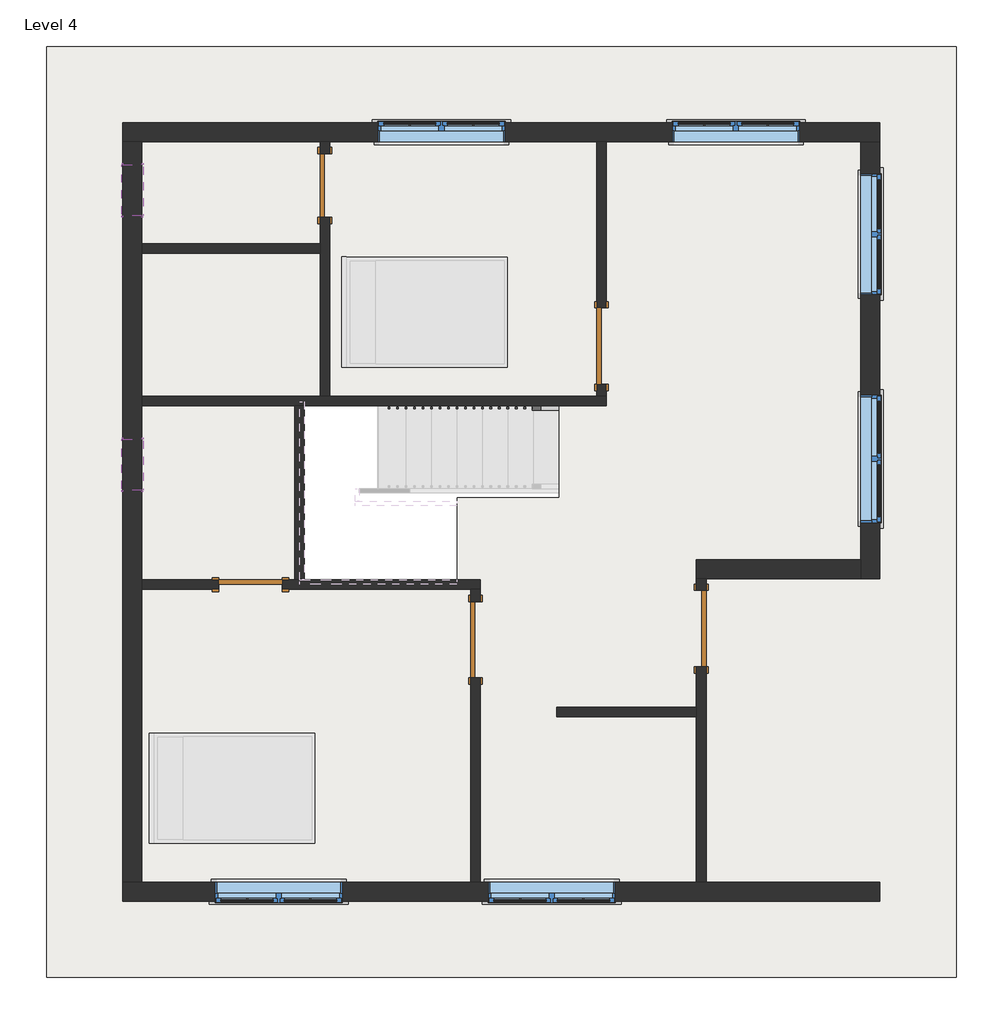
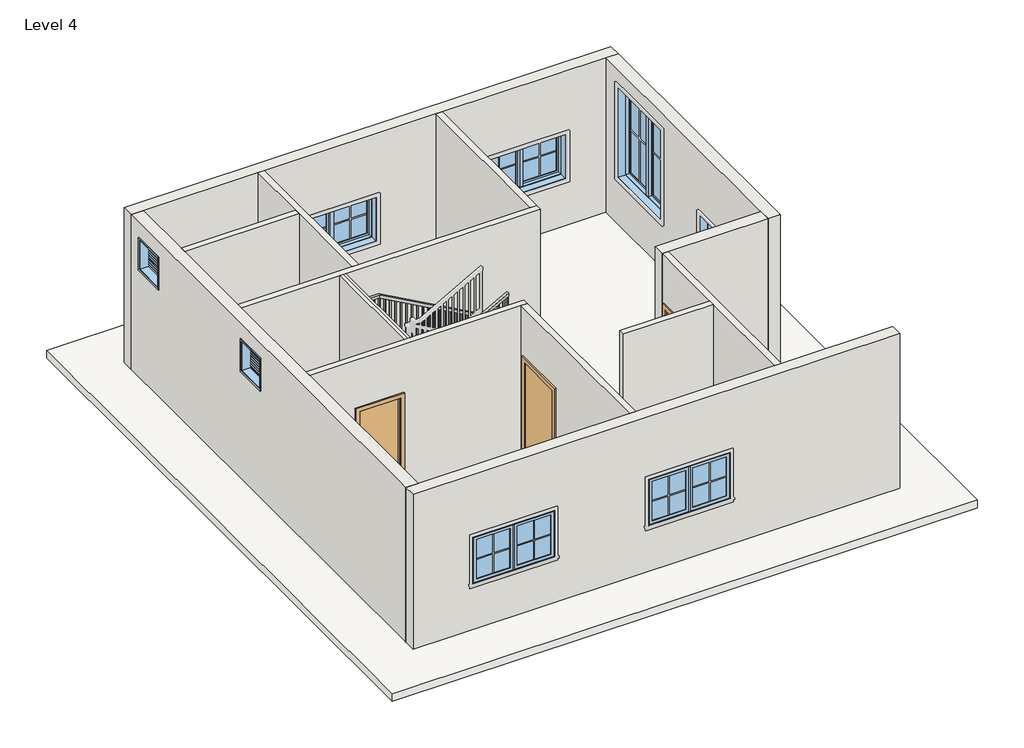
# One storey, part 1 of 2: 14 walls, 8 windows, 5 doors, 1 railing, 1 roof.
# Revit data of these elements (continued)
# Element 23 (IfcWindow, "Window-Casement-Double : WINDOW 6\"") (continued)
#   Interior Wall Closure = 0' - 2 1/4"
#   Frame Extension = 0' - 0 1/4"
#   Exterior Wall Closure = 0' - 1 1/4"
#   Interior Trim Visibility = yes
#   Exterior Trim Visibility = yes
#   Phase Created = New Construction
#   Materials on its faces: "Wood - Stained", "Glass", "Clad - White"
# Element 24 (IfcWindow, "Window-Casement-Double : WINDOW 6\"")
#   Mark = "26"
#   Window Inset = 0' - 0"
#   Interior Wall Closure = 0' - 2 1/4"
#   Frame Extension = 0' - 0 1/4"
#   Exterior Wall Closure = 0' - 1 1/4"
#   Interior Trim Visibility = yes
#   Exterior Trim Visibility = yes
#   Phase Created = New Construction
#   Materials on its faces: "Wood - Stained", "Glass", "Clad - White"
# Element 25 (IfcWindow, "Window-Casement-Double : WINDOW 6\"")
#   Mark = "27"
#   Window Inset = 0' - 0"
#   Interior Wall Closure = 0' - 2 1/4"
#   Frame Extension = 0' - 0 1/4"
#   Exterior Wall Closure = 0' - 1 1/4"
#   Interior Trim Visibility = yes
#   Exterior Trim Visibility = yes
#   Phase Created = New Construction
#   Materials on its faces: "Wood - Stained", "Glass", "Clad - White"
# Element 26 (IfcWindow, "Window-Casement-Double : WINDOW 6\"")
#   Mark = "28"
#   Window Inset = 0' - 0"
#   Interior Wall Closure = 0' - 2 1/4"
#   Frame Extension = 0' - 0 1/4"
#   Exterior Wall Closure = 0' - 1 1/4"
#   Interior Trim Visibility = yes
#   Exterior Trim Visibility = yes
#   Phase Created = New Construction
#   Materials on its faces: "Wood - Stained", "Glass", "Clad - White"
# Element 27 (IfcWindow, "Window-Casement-Double : WINDOW 6\"")
#   Mark = "29"
#   Window Inset = 0' - 0"
#   Interior Wall Closure = 0' - 2 1/4"
#   Frame Extension = 0' - 0 1/4"
#   Exterior Wall Closure = 0' - 1 1/4"
#   Interior Trim Visibility = yes
#   Exterior Trim Visibility = yes
#   Phase Created = New Construction
#   Materials on its faces: "Wood - Stained", "Glass", "Clad - White"
# Element 28 (IfcWindow, "Window-Louvers : 24\" x 24\"")
#   Mark = "30"
#   Blade Width = 1' - 10 1/2"
#   Phase Created = New Construction
#   Materials on its faces: "Birch"
# Element 29 (IfcWindow, "Window-Louvers : 24\" x 24\"")
#   Mark = "31"
#   Blade Width = 1' - 10 1/2"
#   Phase Created = New Construction
#   Materials on its faces: "Birch"
# Materials
#   "Door - Panel": class "Wood", colour RGB 210 159 95, transparency 0, Cost = 0
#   "Door - Frame": colour RGB 118 70 51, transparency 0, Cost = 0
#   "Wood - Stained": class "Wood", colour RGB 224 178 126, transparency 0, Cost = 0
#   "Glass": class "Glass", colour RGB 0 128 192, transparency 0.75, Description = "Soda Lime Glass", Cost = 0
#   "Clad - White": class "Wood", colour RGB 242 242 238, transparency 0, Cost = 0
#   "Birch": class "Wood", colour RGB 224 178 126, transparency 0, Description = "Betula Alleghaniensis", Cost = 0
#   "Default Wall": colour RGB 128 128 128, transparency 0, Cost = 0
